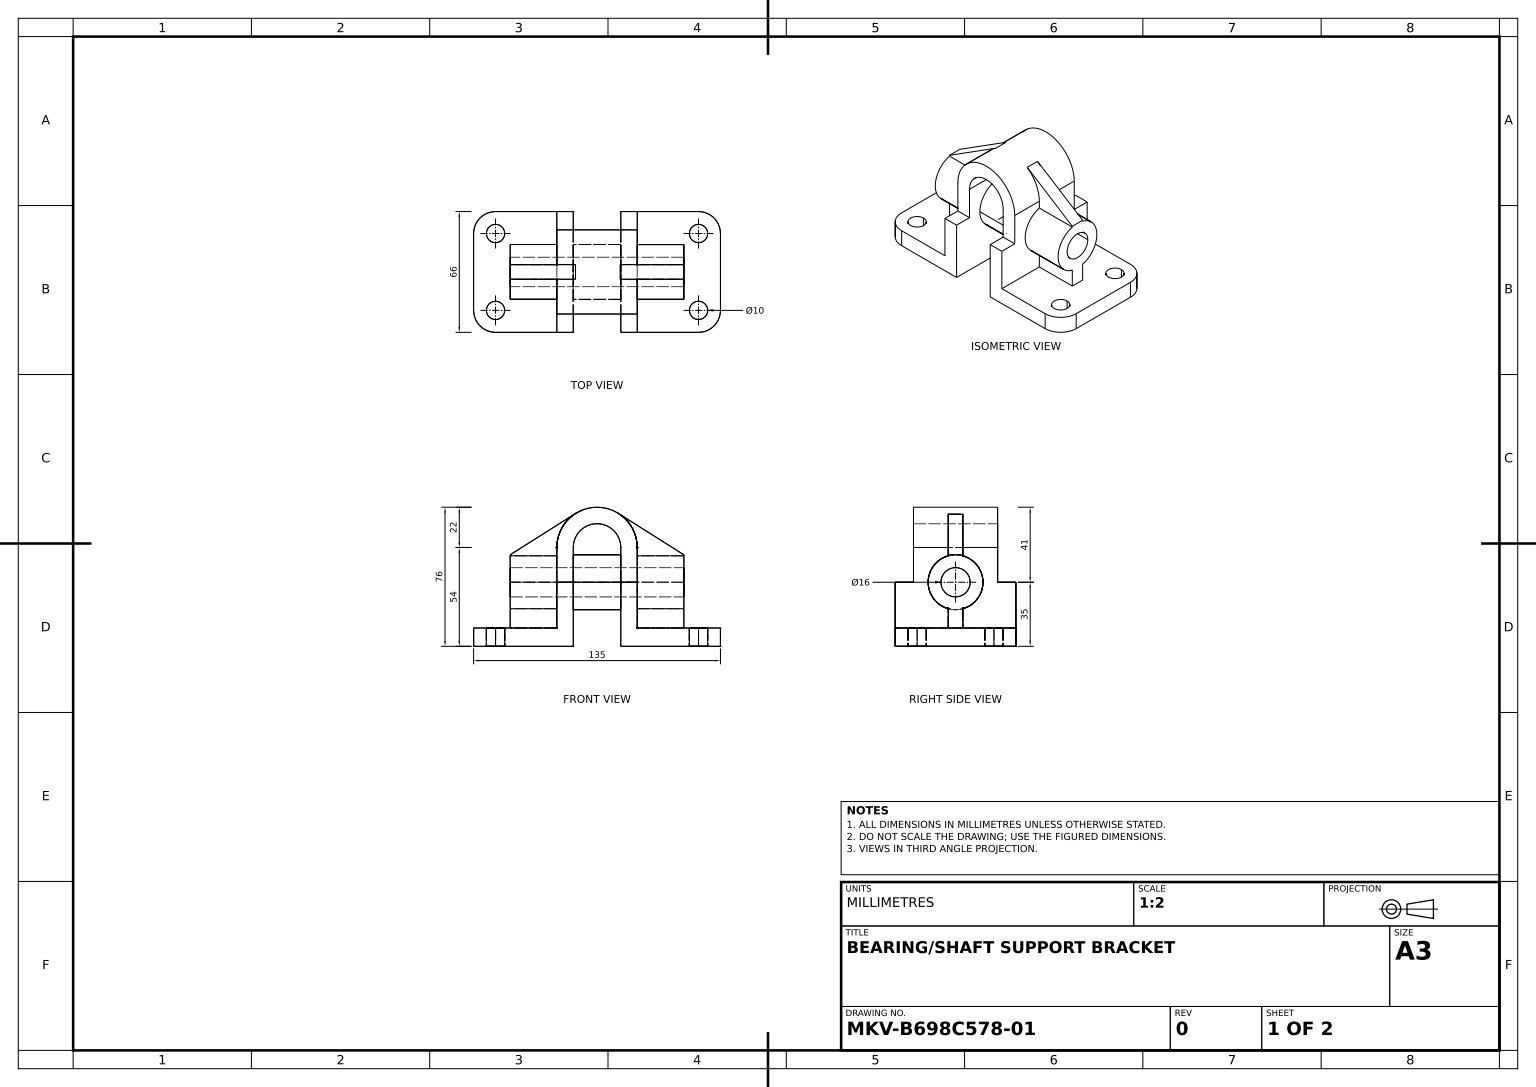
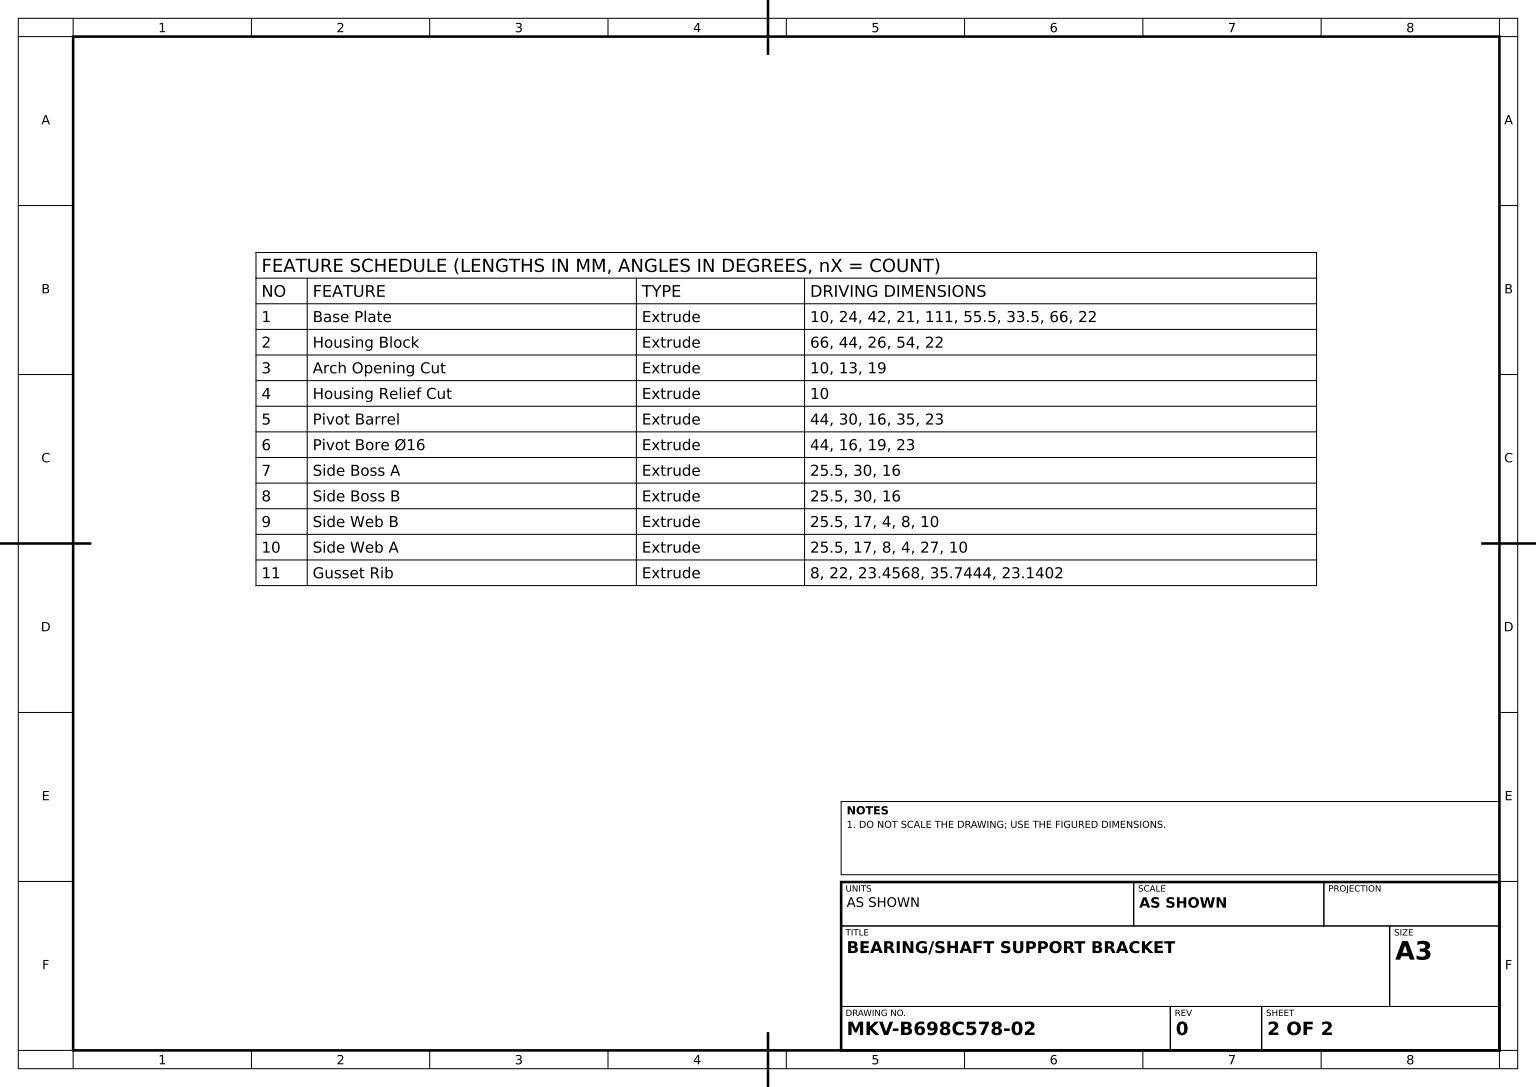
from build123d import *

# Parameters (mm, degrees)
BASE_PLATE_SKETCH_R      = 5
BASE_PLATE_DEPTH         = 10
BASE_PLATE_2_DEPTH       = 10
HOUSING_BLOCK_DEPTH      = 66
ARCH_OPENING_CUT_DEPTH   = 10
HOUSING_START            = -10
HOUSING_RELIEF_CUT_DEPTH = 10
PIVOT_BARREL_SKETCH_R    = 15
PIVOT_BARREL_SKETCH_R_2  = 8
PIVOT_BARREL_DEPTH       = 44
PIVOT_BORE_SKETCH_R      = 8
PIVOT_BORE_16_DEPTH      = 44
SIDE_START               = 25.5
SIDE_BOSS_A_SKETCH_R     = 15
SIDE_BOSS_A_SKETCH_R_2   = 8
SIDE_BOSS_A_DEPTH        = 25.5
SIDE_BOSS_B_SKETCH_R     = 15
SIDE_BOSS_B_SKETCH_R_2   = 8
SIDE_BOSS_B_DEPTH        = 25.5
SIDE_WEB_B_SKETCH_W      = 8
SIDE_WEB_B_SKETCH_H      = 17
SIDE_WEB_B_DEPTH         = 25.5
SIDE_WEB_A_SKETCH_W      = 8
SIDE_WEB_A_SKETCH_H      = 17
SIDE_WEB_A_DEPTH         = 25.5
GUSSET_RIB_DEPTH         = 4


with BuildPart() as part:
    # Base Plate Sketch → Base Plate (new body)
    with BuildSketch(Plane(origin=(0, 0, 0), x_dir=(1, 0, 0), z_dir=(0, 1, 0))):
        with BuildLine():
            Line((-55.5, 33), (-22, 33))
            Line((-22, 33), (-22, -33))
            Line((-22, -33), (-55.5, -33))
            ThreePointArc((-55.5, -33), (-63.985281374, -29.485281374), (-67.5, -21))
            Line((-67.5, -21), (-67.5, 21))
            ThreePointArc((-67.5, 21), (-63.985281374, 29.485281374), (-55.5, 33))
        make_face()
        with Locations(Location((-55.5, 21, 0), (0, 0, 270))):
            Circle(BASE_PLATE_SKETCH_R, mode=Mode.SUBTRACT)
        with Locations(Location((-55.5, -21, 0), (0, 0, 270))):
            Circle(BASE_PLATE_SKETCH_R, mode=Mode.SUBTRACT)
    extrude(amount=BASE_PLATE_DEPTH)



with BuildPart() as body_2:
    # Base Plate Sketch → Base Plate 2 (new body)
    with BuildSketch(Plane(origin=(0, 0, 0), x_dir=(1, 0, 0), z_dir=(0, 1, 0))):
        with BuildLine():
            Line((67.5, 21), (67.5, -21))
            ThreePointArc((67.5, -21), (63.985281374, -29.485281374), (55.5, -33))
            Line((55.5, -33), (22, -33))
            Line((22, -33), (22, 33))
            Line((22, 33), (55.5, 33))
            ThreePointArc((55.5, 33), (63.985281374, 29.485281374), (67.5, 21))
        make_face()
        with Locations(Location((55.5, 21, 0), (0, 0, 270))):
            Circle(BASE_PLATE_SKETCH_R, mode=Mode.SUBTRACT)
        with Locations(Location((55.5, -21, 0), (0, 0, 270))):
            Circle(BASE_PLATE_SKETCH_R, mode=Mode.SUBTRACT)
    extrude(amount=BASE_PLATE_2_DEPTH)


with BuildPart() as part_1:
    add(part.part)

    add(body_2.part)  # Housing Block merges body 2
    # Housing Block Sketch → Housing Block (add)
    with BuildSketch(Plane.XY.offset(33)):
        with BuildLine():
            Line((-22, 54), (-22, 10))
            Line((-22, 10), (-22, 0))
            Line((-22, 0), (-13, 0))
            Line((-13, 0), (-13, 54))
            ThreePointArc((-13, 54), (0, 67), (13, 54))
            Line((13, 54), (13, 0))
            Line((13, 0), (22, 0))
            Line((22, 0), (22, 54))
            ThreePointArc((22, 54), (0, 76), (-22, 54))
        make_face()
    extrude(amount=-HOUSING_BLOCK_DEPTH)

    # Arch Opening Sketch → Arch Opening Cut (cut)
    with BuildSketch(Plane.XY.offset(33)):
        with BuildLine():
            Line((13, 54), (13, 35))
            Line((13, 35), (22, 35))
            Line((22, 35), (22, 54))
            ThreePointArc((22, 54), (0, 76), (-22, 54))
            Line((-22, 54), (-22, 35))
            Line((-22, 35), (-13, 35))
            Line((-13, 35), (-13, 54))
            ThreePointArc((-13, 54), (0, 67), (13, 54))
        make_face()
    extrude(amount=-ARCH_OPENING_CUT_DEPTH, mode=Mode.SUBTRACT)

    # Housing Relief Sketch → Housing Relief Cut (cut)
    with BuildSketch(Plane(origin=(0, 0, -33), x_dir=(-1, 0, 0), z_dir=(0, 0, -1)).offset(HOUSING_START)):
        with BuildLine():
            Line((-13, 35), (-22, 35))
            Line((-22, 35), (-22, 54))
            ThreePointArc((-22, 54), (0, 76), (22, 54))
            Line((22, 54), (22, 35))
            Line((22, 35), (13, 35))
            Line((13, 35), (13, 54))
            ThreePointArc((13, 54), (0, 67), (-13, 54))
            Line((-13, 54), (-13, 35))
        make_face()
    extrude(amount=HOUSING_RELIEF_CUT_DEPTH, mode=Mode.SUBTRACT)

    # Pivot Barrel Sketch → Pivot Barrel (add)
    with BuildSketch(Plane.ZY.offset(22)):
        with Locations((0, 35)):
            Circle(PIVOT_BARREL_SKETCH_R)
        with Locations((0, 35)):
            Circle(PIVOT_BARREL_SKETCH_R_2, mode=Mode.SUBTRACT)
    extrude(amount=-PIVOT_BARREL_DEPTH)

    # Pivot Bore Sketch → Pivot Bore Ø16 (cut)
    with BuildSketch(Plane.ZY.offset(22)):
        with Locations((0, 35)):
            Circle(PIVOT_BORE_SKETCH_R)
    extrude(amount=-PIVOT_BORE_16_DEPTH, mode=Mode.SUBTRACT)

    # Side Boss A Sketch → Side Boss A (add)
    with BuildSketch(Plane.ZY.offset(22).offset(SIDE_START)):
        with Locations((0, 35)):
            Circle(SIDE_BOSS_A_SKETCH_R)
        with Locations((0, 35)):
            Circle(SIDE_BOSS_A_SKETCH_R_2, mode=Mode.SUBTRACT)
    extrude(amount=-SIDE_BOSS_A_DEPTH)

    # Side Boss B Sketch → Side Boss B (add)
    with BuildSketch(Plane(origin=(22, 0, 0), x_dir=(0, 0, -1), z_dir=(1, 0, 0))):
        with Locations(Location((0, 35, 0), (0, 0, 180))):
            Circle(SIDE_BOSS_B_SKETCH_R)
        with Locations(Location((0, 35, 0), (0, 0, 180))):
            Circle(SIDE_BOSS_B_SKETCH_R_2, mode=Mode.SUBTRACT)
    extrude(amount=SIDE_BOSS_B_DEPTH)

    # Side Web B Sketch → Side Web B (add)
    with BuildSketch(Plane(origin=(47.5, 0, 0), x_dir=(0, 0, -1), z_dir=(1, 0, 0))):
        with Locations((0, 18.5)):
            Rectangle(SIDE_WEB_B_SKETCH_W, SIDE_WEB_B_SKETCH_H)
    extrude(amount=-SIDE_WEB_B_DEPTH)

    # Side Web A Sketch → Side Web A (add)
    with BuildSketch(Plane.ZY.offset(47.5)):
        with Locations((0, 18.5)):
            Rectangle(SIDE_WEB_A_SKETCH_W, SIDE_WEB_A_SKETCH_H)
    extrude(amount=-SIDE_WEB_A_DEPTH)

    # Gusset Rib Sketch → Gusset Rib (add, symmetric)
    with BuildSketch(Plane.XY):
        with BuildLine():
            Line((-11.755648115, 72.595825806), (-47.5, 50))
            Line((-47.5, 50), (-47.5, 44))
            Line((-47.5, 44), (-22, 44))
            Line((-22, 44), (-22, 54))
            ThreePointArc((-22, 54), (-19.269461053, 64.615454335), (-11.755648115, 72.595825806))
        make_face()
        with BuildLine():
            Line((47.5, 50), (12.615670058, 72.023453304))
            ThreePointArc((12.615670058, 72.023453304), (19.513389522, 64.16009987), (22, 54))
            Line((22, 54), (22, 44))
            Line((22, 44), (47.5, 44))
            Line((47.5, 44), (47.5, 50))
        make_face()
    extrude(amount=GUSSET_RIB_DEPTH, both=True)


solid = part_1.part
